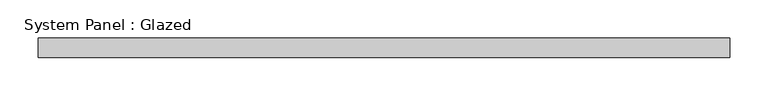
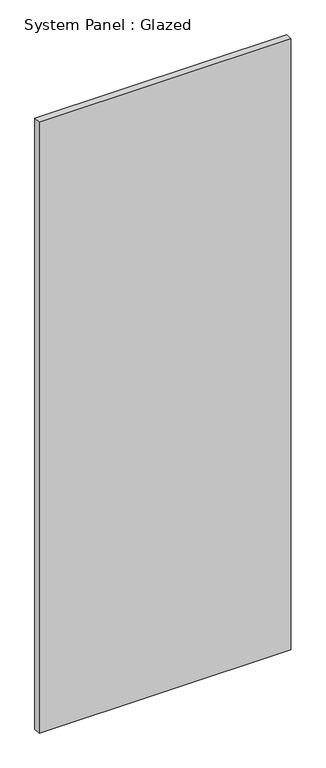
"""IFC4 building model written with IfcOpenShell, lengths in millimetres: plate geometry, System Panel : Glazed."""

from ifc_helpers import new_model, si_unit, origin, origin_with_axes, place, context, project, spatial, polyline, outline, extrude, source, transform, mapped, element, save


def system_panel_glazed_85e9b79d(model_context):
    return source(origin(), model_context, "Body", "SweptSolid", [
        extrude(outline(polyline([(450.85, 19.05), (-450.85, 19.05), (-450.85, 44.45), (450.85, 44.45), (450.85, 19.05)])), origin_with_axes(), (0.0, 0.0, 1.0), 2313.0217298),
    ])


if __name__ == "__main__":
    model = new_model("IFC4")
    model_context = context("Model", 3, world=origin())
    ifc_project = project(units=[si_unit("LENGTHUNIT", "METRE", prefix="MILLI")], contexts=[model_context])
    site = spatial("IfcSite", under=ifc_project)
    building = spatial("IfcBuilding", under=site)
    placement = place(None, origin())
    system_panel_glazed_shape = system_panel_glazed_85e9b79d(model_context)
    element("IfcPlate", 1, ObjectType="System Panel : Glazed", at=placement, inside=building, context=model_context, shape_type="MappedRepresentation", body=[
        mapped(system_panel_glazed_shape, transform((0.0, 0.0, 0.0), x_axis=(1.0, 0.0, 0.0), y_axis=(0.0, 1.0, 0.0), z_axis=(0.0, 0.0, 1.0))),
    ])
    save(model, "model.ifc")

# Revit data of these elements
# Type "System Panel : Glazed"
#   Construction Type Id = "GSP4R"
#   Analytic Construction = "1/8 in Pilkington single glazing"
#   Visual Light Transmittance = 0.9
#   Solar Heat Gain Coefficient = 0.86
#   Heat Transfer Coefficient (U) = 1.18115 BTU/(h·ft²·°F)
#   Define Thermal Properties by = 1
# Element 1 (IfcPlate, "System Panel : Glazed")
#   Materials on its faces: "Glass"
# Materials
#   "Glass": class "Glass", colour RGB 0 128 192, transparency 0.75, Description = "Soda Lime Glass", Cost = 0
